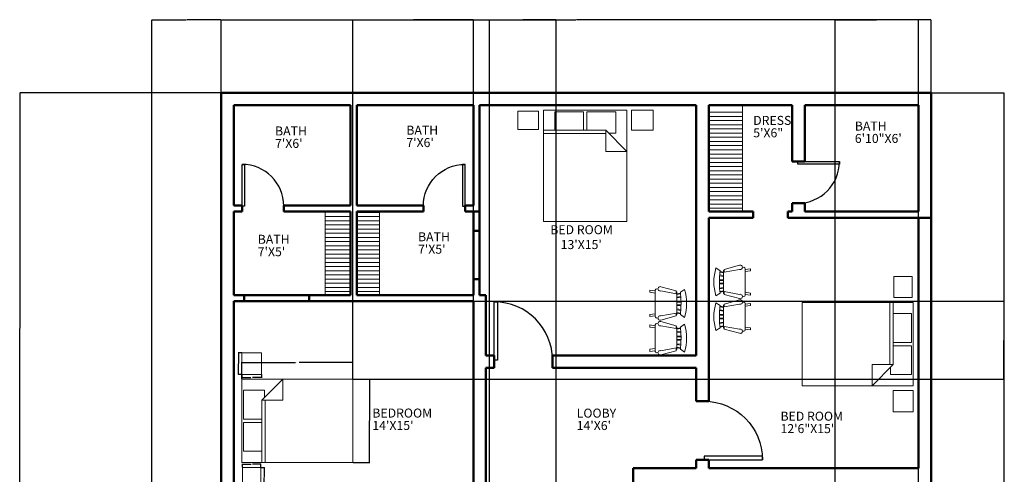
# Model space of a CAD drawing. Units: inches. Extents: x 5375 to 6084, y 16106 to 17259.
# Tile 32 of 32: x 5376 to 6084, y 16932 to 17259. Entities that reach past the tile are written whole.
import ezdxf

# ---------------------------------------------------------------- set-up
doc = ezdxf.new("R2010")
doc.units = ezdxf.units.IN
for name, color, linetype, lineweight in [('A-ANNO-DIMS', 2, 'Continuous', 18), ('A-AREA-IDEN', 5, 'Continuous', 18), ('A-CASE-PATT', 3, 'Continuous', 13), ('A-FLOR-CASE', 3, 'Continuous', 18), ('DOOR', 4, 'Continuous', 25), ('FURNITURE', 3, 'Continuous', 18), ('WALL', 6, 'Continuous', 50)]:
    doc.layers.add(name, color=color, linetype=linetype, lineweight=lineweight)
doc.styles.get("Standard").update_dxf_attribs({"font": 'arial.ttf'})
doc.dimstyles.get("Standard").update_dxf_attribs({"dimtxt": 0.18, "dimasz": 0.18, "dimexe": 0.18, "dimexo": 0.0625, "dimgap": 0.09, "dimtad": 0, "dimtih": 1, "dimtoh": 1, "dimdec": 4, "dimzin": 0, "dimdsep": 46, "dimtxsty": 'Standard', "dimcen": 0.09, "dimadec": 0, "dimazin": 0, "dimtfac": 1, "dimtdec": 4, "dimtofl": 0, "dimtmove": 0, "dimatfit": 3, "dimfxl": 1, "dimtolj": 1, "dimtzin": 0, "dimarcsym": 0})

# ---------------------------------------------------------------- blocks, each defined once
blk = doc.blocks.new('*U2')
for p, q in [((0, 0), (0, -100)), ((750, 0), (750, -100))]:
    blk.add_line(p, q)
blk.add_lwpolyline([(0, 0), (0, 750), (43.75, 750), (43.75, 0)], close=True)
blk.add_arc((0, 0), 750, 0, 90)
blk = doc.blocks.new('Bed - Queen')
for p, q in [((0, -80.00003), (0, 0)), ((0, 0), (59.99999, 0)), ((59.99999, 0), (59.99999, -80.00003)), ((7.99999, -1.2), (28.79998, -1.2)), ((7.99999, -14.4), (7.99999, -1.2)), ((28.79998, -1.2), (28.79998, -14.4)), ((31.19999, -1.2), (51.99999, -1.2)), ((31.19999, -14.4), (31.19999, -1.2)), ((51.99999, -1.2), (51.99999, -16.4)), ((0, -14.4), (44.8, -14.4)), ((44.8, -16.8), (0, -16.8)), ((59.99999, -29.6), (44.8, -14.4)), ((44.8, -14.4), (44.8, -29.6)), ((51.99999, -16.4), (46.79936, -16.4)), ((44.8, -29.6), (59.99999, -29.6)), ((59.99999, -80.00003), (0, -80.00003))]:
    blk.add_line(p, q)
blk = doc.blocks.new('Chair - Rocking')
for p, q in [((-8, -4.5), (-10, -1.5)), ((-8.23428, -6.99939), (-8.3093, -7.47958)), ((-8.23041, -7), (8.23915, -7)), ((-7.5, -4.5), (-7, -7)), ((-6.5, -7), (-7.02225, -4.43)), ((-4.5, -7), (-4.96674, -4.19951)), ((-4, -7), (-4.40532, -4.16272)), ((-1.5, -4.05012), (-1.5, -7)), ((-1, -7), (-1, -4.05012)), ((1, -7), (1, -4.04655)), ((1.5, -4.05012), (1.5, -7)), ((4, -7), (4.40187, -4.18694)), ((4.5, -7), (4.96761, -4.19437)), ((6.5, -7), (7, -4.4057)), ((7.5, -4.5), (7, -7)), ((8, -4.5), (10, -1.5)), ((8.31071, -7.48854), (8.23449, -7.00073)), ((-9, -7.5), (-12, -18.49999)), ((-7, -7.5), (-9, -7.5)), ((-9, -18.49999), (-7, -7.5)), ((7, -7.5), (9, -7.5)), ((9, -18.49999), (7, -7.5)), ((9, -7.5), (12, -18.49999)), ((-10.36644, -20.64523), (-10.5, -21.49999)), ((10.5, -21.49999), (10.3575, -20.58798)), ((-9, -22.49999), (-9.5, -26.49999)), ((0, -22.49999), (-9.5, -22.49999)), ((-9.5, -26.49999), (-8, -26.49999)), ((-8, -26.49999), (-7.5, -22.49999)), ((0, -22.49999), (9.5, -22.49999)), ((8, -26.49999), (7.5, -22.49999)), ((9.5, -26.49999), (8, -26.49999)), ((9, -22.49999), (9.5, -26.49999))]:
    blk.add_line(p, q)
for centre, radius, start, end in [((0, -34.08333), 34.08333, 72.93847, 107.0615), ((0, -68.25004), 64.25, 93.92211, 97.15267), ((0, -68.25004), 64.25, 82.84733, 93.92211), ((-10.5, -18.99999), 1.58114, 161.5651, 18.43495), ((10.5, -18.99999), 1.58114, 161.5651, 18.43495), ((-9.5, -21.49999), 1, 180, 270), ((9.5, -21.49999), 1, 270, 0)]:
    blk.add_arc(centre, radius, start, end)
blk = doc.blocks.new('NIGHTSTAND-SMALL')
blk.add_lwpolyline([(0, 13.23), (15.04, 13.23), (15.04, 0), (0, 0)], close=True)
blk = doc.blocks.new('NIGHTSTAND-LARGE')
blk.add_lwpolyline([(0, 14.27), (15.49, 14.27), (15.49, 0), (0, 0)], close=True)
blk = doc.blocks.new('*D16')
at = {"layer": 'A-ANNO-DIMS', "color": 0, "lineweight": -2, "transparency": 16777216}
for p, q in [((5535.35, 17019.44), (5532.91, 17019.44)), ((5533.09, 17019.26), (5533.09, 17011.88)), ((5533.09, 17004.13), (5533.09, 17011.52)), ((5535.35, 17003.95), (5532.91, 17003.95))]:
    blk.add_line(p, q, dxfattribs=at)
at = {"layer": 'A-ANNO-DIMS', "color": 0, "transparency": 16777216}
for points in [[(5533.06, 17019.26), (5533.12, 17019.26), (5533.09, 17019.44)], [(5533.06, 17004.13), (5533.12, 17004.13), (5533.09, 17003.95)]]:
    blk.add_solid(points, dxfattribs=at)
at = {"layer": 'Defpoints', "color": 0, "transparency": 16777216}
for p in [(5533.09, 17019.44), (5535.41, 17019.44), (5535.41, 17003.95)]:
    blk.add_point(p, dxfattribs=at)
at = {"layer": 'A-ANNO-DIMS', "color": 0, "transparency": 16777216, "insert": (5533.09, 17011.7), "char_height": 0.18, "attachment_point": 5}
blk.add_mtext('\\A1;LG. NIGHTSTAND 15 TYP.', dxfattribs=at)
blk = doc.blocks.new('*D17')
at = {"layer": 'A-ANNO-DIMS', "color": 0, "lineweight": -2, "transparency": 16777216}
for p, q in [((5535.41, 17003.89), (5535.41, 17001.45)), ((5549.68, 17003.89), (5549.68, 17001.45)), ((5535.59, 17001.63), (5542.03, 17001.63)), ((5549.5, 17001.63), (5543.07, 17001.63))]:
    blk.add_line(p, q, dxfattribs=at)
at = {"layer": 'A-ANNO-DIMS', "color": 0, "transparency": 16777216}
for points in [[(5535.59, 17001.66), (5535.59, 17001.6), (5535.41, 17001.63)], [(5549.5, 17001.66), (5549.5, 17001.6), (5549.68, 17001.63)]]:
    blk.add_solid(points, dxfattribs=at)
at = {"layer": 'Defpoints', "color": 0, "transparency": 16777216}
for p in [(5535.41, 17003.95), (5549.68, 17003.95), (5535.41, 17001.63)]:
    blk.add_point(p, dxfattribs=at)
at = {"layer": 'A-ANNO-DIMS', "color": 0, "transparency": 16777216, "insert": (5542.55, 17001.63), "char_height": 0.18, "attachment_point": 5}
blk.add_mtext('\\A1;14 TYP.', dxfattribs=at)
blk = doc.blocks.new('*D18')
at = {"layer": 'A-ANNO-DIMS', "color": 0, "lineweight": -2, "transparency": 16777216}
for p, q in [((5549.3, 16937.05), (5551.67, 16937.05)), ((5551.49, 16936.87), (5551.49, 16929.72)), ((5551.49, 16922.19), (5551.49, 16929.35)), ((5549.3, 16922.01), (5551.67, 16922.01))]:
    blk.add_line(p, q, dxfattribs=at)
at = {"layer": 'A-ANNO-DIMS', "color": 0, "transparency": 16777216}
for points in [[(5551.46, 16936.87), (5551.52, 16936.87), (5551.49, 16937.05)], [(5551.46, 16922.19), (5551.52, 16922.19), (5551.49, 16922.01)]]:
    blk.add_solid(points, dxfattribs=at)
at = {"layer": 'Defpoints', "color": 0, "transparency": 16777216}
for p in [(5549.24, 16937.05), (5551.49, 16937.05), (5549.24, 16922.01)]:
    blk.add_point(p, dxfattribs=at)
at = {"layer": 'A-ANNO-DIMS', "color": 0, "transparency": 16777216, "insert": (5551.49, 16929.53), "char_height": 0.18, "attachment_point": 5}
blk.add_mtext('\\A1;SM. NIGHTSTAND 15 TYP.', dxfattribs=at)
blk = doc.blocks.new('*D19')
at = {"layer": 'A-ANNO-DIMS', "color": 0, "lineweight": -2, "transparency": 16777216}
for p, q in [((5536.01, 16937.12), (5536.01, 16939.49)), ((5536.19, 16939.31), (5542.1, 16939.31)), ((5549.06, 16939.31), (5543.14, 16939.31)), ((5549.24, 16937.12), (5549.24, 16939.49))]:
    blk.add_line(p, q, dxfattribs=at)
at = {"layer": 'A-ANNO-DIMS', "color": 0, "transparency": 16777216}
for points in [[(5536.19, 16939.34), (5536.19, 16939.28), (5536.01, 16939.31)], [(5549.06, 16939.34), (5549.06, 16939.28), (5549.24, 16939.31)]]:
    blk.add_solid(points, dxfattribs=at)
at = {"layer": 'Defpoints', "color": 0, "transparency": 16777216}
for p in [(5536.01, 16939.31), (5536.01, 16937.05), (5549.24, 16937.05)]:
    blk.add_point(p, dxfattribs=at)
at = {"layer": 'A-ANNO-DIMS', "color": 0, "transparency": 16777216, "insert": (5542.62, 16939.31), "char_height": 0.18, "attachment_point": 5}
blk.add_mtext('\\A1;13 TYP.', dxfattribs=at)
blk = doc.blocks.new('*D20')
at = {"layer": 'A-ANNO-DIMS', "color": 0, "lineweight": -2, "transparency": 16777216}
for p, q in [((5535.41, 17000.67), (5535.41, 17012.79)), ((5535.59, 17012.61), (5574.11, 17012.61)), ((5615.23, 17012.61), (5576.72, 17012.61)), ((5615.41, 17000.67), (5615.41, 17012.79))]:
    blk.add_line(p, q, dxfattribs=at)
at = {"layer": 'A-ANNO-DIMS', "color": 0, "transparency": 16777216}
for points in [[(5535.59, 17012.64), (5535.59, 17012.58), (5535.41, 17012.61)], [(5615.23, 17012.64), (5615.23, 17012.58), (5615.41, 17012.61)]]:
    blk.add_solid(points, dxfattribs=at)
at = {"layer": 'Defpoints', "color": 0, "transparency": 16777216}
for p in [(5535.41, 17012.61), (5535.41, 17000.61), (5615.41, 17000.61)]:
    blk.add_point(p, dxfattribs=at)
at = {"layer": 'A-ANNO-DIMS', "color": 0, "transparency": 16777216, "insert": (5575.41, 17012.61), "char_height": 0.18, "attachment_point": 5}
blk.add_mtext('\\A1;QUEEN BED 80 TYP.', dxfattribs=at)
blk = doc.blocks.new('*D21')
at = {"layer": 'A-ANNO-DIMS', "color": 0, "lineweight": -2, "transparency": 16777216}
for p, q in [((5615.48, 17000.61), (5627.59, 17000.61)), ((5627.41, 17000.43), (5627.41, 16970.79)), ((5627.41, 16940.79), (5627.41, 16970.43)), ((5615.48, 16940.61), (5627.59, 16940.61))]:
    blk.add_line(p, q, dxfattribs=at)
at = {"layer": 'A-ANNO-DIMS', "color": 0, "transparency": 16777216}
for points in [[(5627.38, 17000.43), (5627.44, 17000.43), (5627.41, 17000.61)], [(5627.38, 16940.79), (5627.44, 16940.79), (5627.41, 16940.61)]]:
    blk.add_solid(points, dxfattribs=at)
at = {"layer": 'Defpoints', "color": 0, "transparency": 16777216}
for p in [(5615.41, 17000.61), (5627.41, 17000.61), (5615.41, 16940.61)]:
    blk.add_point(p, dxfattribs=at)
at = {"layer": 'A-ANNO-DIMS', "color": 0, "transparency": 16777216, "insert": (5627.41, 16970.61), "char_height": 0.18, "attachment_point": 5}
blk.add_mtext('\\A1;60 TYP.', dxfattribs=at)
blk = doc.blocks.new('*D31')
at = {"layer": 'A-ANNO-DIMS', "color": 0, "lineweight": -2, "transparency": 16777216}
for p, q in [((6031.68, 17206.58), (6084.2, 17206.58)), ((6084.02, 17206.4), (6084.02, 16709.66)), ((6084.02, 16212.56), (6084.02, 16709.3)), ((6031.68, 16212.38), (6084.2, 16212.38))]:
    blk.add_line(p, q, dxfattribs=at)
at = {"layer": 'A-ANNO-DIMS', "color": 0, "transparency": 16777216}
for points in [[(6083.99, 17206.4), (6084.05, 17206.4), (6084.02, 17206.58)], [(6083.99, 16212.56), (6084.05, 16212.56), (6084.02, 16212.38)]]:
    blk.add_solid(points, dxfattribs=at)
at = {"layer": 'Defpoints', "color": 0, "transparency": 16777216}
for p in [(6031.62, 17206.58), (6084.02, 17206.58), (6031.62, 16212.38)]:
    blk.add_point(p, dxfattribs=at)
at = {"layer": 'A-ANNO-DIMS', "color": 0, "transparency": 16777216, "insert": (6084.02, 16709.48), "char_height": 0.18, "attachment_point": 5}
blk.add_mtext('\\A1;994.2', dxfattribs=at)
blk = doc.blocks.new('*D32')
at = {"layer": 'A-ANNO-DIMS', "color": 0, "lineweight": -2, "transparency": 16777216}
for p, q in [((5520.62, 17206.64), (5520.62, 17259.16)), ((6031.62, 17206.64), (6031.62, 17259.16)), ((5520.8, 17258.98), (5775.85, 17258.98)), ((6031.44, 17258.98), (5776.39, 17258.98))]:
    blk.add_line(p, q, dxfattribs=at)
at = {"layer": 'A-ANNO-DIMS', "color": 0, "transparency": 16777216}
for points in [[(5520.8, 17259.01), (5520.8, 17258.95), (5520.62, 17258.98)], [(6031.44, 17259.01), (6031.44, 17258.95), (6031.62, 17258.98)]]:
    blk.add_solid(points, dxfattribs=at)
at = {"layer": 'Defpoints', "color": 0, "transparency": 16777216}
for p in [(6031.62, 17258.98), (5520.62, 17206.58), (6031.62, 17206.58)]:
    blk.add_point(p, dxfattribs=at)
at = {"layer": 'A-ANNO-DIMS', "color": 0, "transparency": 16777216, "insert": (5776.12, 17258.98), "char_height": 0.18, "attachment_point": 5}
blk.add_mtext('\\A1;511', dxfattribs=at)
blk = doc.blocks.new('*D37')
at = {"layer": 'A-ANNO-DIMS', "color": 0, "lineweight": -2, "transparency": 16777216}
for p, q in [((5520.56, 17206.58), (5375.56, 17206.58)), ((5375.74, 17206.4), (5375.74, 17037.26)), ((5375.74, 16867.76), (5375.74, 17036.9)), ((5520.56, 16867.58), (5375.56, 16867.58))]:
    blk.add_line(p, q, dxfattribs=at)
at = {"layer": 'A-ANNO-DIMS', "color": 0, "transparency": 16777216}
for points in [[(5375.71, 17206.4), (5375.77, 17206.4), (5375.74, 17206.58)], [(5375.71, 16867.76), (5375.77, 16867.76), (5375.74, 16867.58)]]:
    blk.add_solid(points, dxfattribs=at)
at = {"layer": 'Defpoints', "color": 0, "transparency": 16777216}
for p in [(5375.74, 17206.58), (5520.62, 17206.58), (5520.62, 16867.58)]:
    blk.add_point(p, dxfattribs=at)
at = {"layer": 'A-ANNO-DIMS', "color": 0, "transparency": 16777216, "insert": (5375.74, 17037.08), "char_height": 0.18, "attachment_point": 5}
blk.add_mtext('\\A1;339', dxfattribs=at)
blk = doc.blocks.new('*D39')
at = {"layer": 'A-ANNO-DIMS', "color": 0, "lineweight": -2, "transparency": 16777216}
for p, q in [((5713.62, 16402.64), (5713.62, 17259.16)), ((5761.62, 16402.64), (5761.62, 17259.16)), ((5713.8, 17258.98), (5737.4, 17258.98)), ((5761.44, 17258.98), (5737.84, 17258.98))]:
    blk.add_line(p, q, dxfattribs=at)
at = {"layer": 'A-ANNO-DIMS', "color": 0, "transparency": 16777216}
for points in [[(5713.8, 17259.01), (5713.8, 17258.95), (5713.62, 17258.98)], [(5761.44, 17259.01), (5761.44, 17258.95), (5761.62, 17258.98)]]:
    blk.add_solid(points, dxfattribs=at)
at = {"layer": 'Defpoints', "color": 0, "transparency": 16777216}
for p in [(5761.62, 17258.98), (5713.62, 16402.58), (5761.62, 16402.58)]:
    blk.add_point(p, dxfattribs=at)
at = {"layer": 'A-ANNO-DIMS', "color": 0, "transparency": 16777216, "insert": (5737.62, 17258.98), "char_height": 0.18, "attachment_point": 5}
blk.add_mtext('\\A1;48', dxfattribs=at)
blk = doc.blocks.new('*D47')
at = {"layer": 'A-ANNO-DIMS', "color": 0, "lineweight": -2, "transparency": 16777216}
for p, q in [((5470.62, 16603.64), (5470.62, 17259.16)), ((5520.62, 17206.64), (5520.62, 17259.16)), ((5470.8, 17258.98), (5495.4, 17258.98)), ((5520.44, 17258.98), (5495.84, 17258.98))]:
    blk.add_line(p, q, dxfattribs=at)
at = {"layer": 'A-ANNO-DIMS', "color": 0, "transparency": 16777216}
for points in [[(5470.8, 17259.01), (5470.8, 17258.95), (5470.62, 17258.98)], [(5520.44, 17259.01), (5520.44, 17258.95), (5520.62, 17258.98)]]:
    blk.add_solid(points, dxfattribs=at)
at = {"layer": 'Defpoints', "color": 0, "transparency": 16777216}
for p in [(5520.62, 17258.98), (5520.62, 17206.58), (5470.62, 16603.58)]:
    blk.add_point(p, dxfattribs=at)
at = {"layer": 'A-ANNO-DIMS', "color": 0, "transparency": 16777216, "insert": (5495.62, 17258.98), "char_height": 0.18, "attachment_point": 5}
blk.add_mtext('\\A1;50', dxfattribs=at)
blk = doc.blocks.new('*D48')
at = {"layer": 'A-ANNO-DIMS', "color": 0, "lineweight": -2, "transparency": 16777216}
for p, q in [((5962.62, 16411.64), (5962.62, 17259.16)), ((6022.62, 16411.64), (6022.62, 17259.16)), ((5962.8, 17258.98), (5992.4, 17258.98)), ((6022.44, 17258.98), (5992.84, 17258.98))]:
    blk.add_line(p, q, dxfattribs=at)
at = {"layer": 'A-ANNO-DIMS', "color": 0, "transparency": 16777216}
for points in [[(5962.8, 17259.01), (5962.8, 17258.95), (5962.62, 17258.98)], [(6022.44, 17259.01), (6022.44, 17258.95), (6022.62, 17258.98)]]:
    blk.add_solid(points, dxfattribs=at)
at = {"layer": 'Defpoints', "color": 0, "transparency": 16777216}
for p in [(6022.62, 17258.98), (5962.62, 16411.58), (6022.62, 16411.58)]:
    blk.add_point(p, dxfattribs=at)
at = {"layer": 'A-ANNO-DIMS', "color": 0, "transparency": 16777216, "insert": (5992.62, 17258.98), "char_height": 0.18, "attachment_point": 5}
blk.add_mtext('\\A1;60', dxfattribs=at)
blk = doc.blocks.new('*D49')
at = {"layer": 'A-ANNO-DIMS', "color": 0, "lineweight": -2, "transparency": 16777216}
for p, q in [((5529.68, 17056.58), (6084.2, 17056.58)), ((6084.02, 17056.4), (6084.02, 17028.78)), ((6084.02, 17000.79), (6084.02, 17028.41)), ((5615.48, 17000.61), (6084.2, 17000.61))]:
    blk.add_line(p, q, dxfattribs=at)
at = {"layer": 'A-ANNO-DIMS', "color": 0, "transparency": 16777216}
for points in [[(6083.99, 17056.4), (6084.05, 17056.4), (6084.02, 17056.58)], [(6083.99, 17000.79), (6084.05, 17000.79), (6084.02, 17000.61)]]:
    blk.add_solid(points, dxfattribs=at)
at = {"layer": 'Defpoints', "color": 0, "transparency": 16777216}
for p in [(5529.62, 17056.58), (5615.41, 17000.61), (6084.02, 17000.61)]:
    blk.add_point(p, dxfattribs=at)
at = {"layer": 'A-ANNO-DIMS', "color": 0, "transparency": 16777216, "insert": (6084.02, 17028.59), "char_height": 0.18, "attachment_point": 5}
blk.add_mtext('\\A1;55.97', dxfattribs=at)
blk = doc.blocks.new('*D50')
at = {"layer": 'A-ANNO-DIMS', "color": 0, "lineweight": -2, "transparency": 16777216}
for p, q in [((5615.41, 17000.67), (5615.41, 17259.16)), ((5702.12, 17056.64), (5702.12, 17259.16)), ((5615.59, 17258.98), (5658.44, 17258.98)), ((5701.94, 17258.98), (5659.09, 17258.98))]:
    blk.add_line(p, q, dxfattribs=at)
at = {"layer": 'A-ANNO-DIMS', "color": 0, "transparency": 16777216}
for points in [[(5615.59, 17259.01), (5615.59, 17258.95), (5615.41, 17258.98)], [(5701.94, 17259.01), (5701.94, 17258.95), (5702.12, 17258.98)]]:
    blk.add_solid(points, dxfattribs=at)
at = {"layer": 'Defpoints', "color": 0, "transparency": 16777216}
for p in [(5702.12, 17258.98), (5702.12, 17056.58), (5615.41, 17000.61)]:
    blk.add_point(p, dxfattribs=at)
at = {"layer": 'A-ANNO-DIMS', "color": 0, "transparency": 16777216, "insert": (5658.77, 17258.98), "char_height": 0.18, "attachment_point": 5}
blk.add_mtext('\\A1;86.7', dxfattribs=at)

msp = doc.modelspace()

# ---------------------------------------------------------------- hatches: boundary and pattern name
at = {"layer": 'A-CASE-PATT'}
h = msp.add_hatch(dxfattribs=at)
h.set_pattern_fill('ANSI31', color=256, scale=0.944856, angle=-45, style=0)
h.paths.add_polyline_path([(5871.6199, 17122.0277), (5895.7926, 17122.0277), (5895.7926, 17194.0277), (5871.6199, 17194.0277)])
h = msp.add_hatch(dxfattribs=at)
h.set_pattern_fill('ANSI31', color=256, scale=0.9448558, angle=-45, style=0)
h.paths.add_polyline_path([(5595.4235, 17062.046), (5613.6199, 17062.046), (5613.6199, 17119.0277), (5595.4235, 17119.0277)])
h = msp.add_hatch(dxfattribs=at)
h.set_pattern_fill('ANSI31', color=256, scale=0.9448558, angle=-45, style=0)
h.paths.add_polyline_path([(5618.1199, 17061.5998), (5634.4811, 17061.5998), (5634.4811, 17121.0793), (5618.1199, 17121.0793)])

# ---------------------------------------------------------------- linework, layer by layer
at = {"layer": 'A-FLOR-CASE'}
for p, q in [((5895.7926, 17121.0793), (5895.7926, 17197.5793)), ((5595.4235, 17061.0793), (5595.4235, 17121.0793)), ((5634.4811, 17061.0793), (5634.4811, 17121.0793))]:
    msp.add_line(p, q, dxfattribs=at)
at = {"layer": 'WALL'}
for p, q in [((5520.6199, 17206.5793), (6031.6199, 17206.5793)), ((5520.6199, 17206.5793), (5520.6199, 16867.5793)), ((6031.6199, 17206.5793), (6031.6199, 16921.5793)), ((5529.6199, 17197.5793), (5613.6199, 17197.5793)), ((5529.6199, 17197.5793), (5529.6199, 17125.5793)), ((5613.6199, 17197.5793), (5613.6199, 17125.5793)), ((5618.1199, 17197.5793), (5618.1199, 17125.5793)), ((5618.1199, 17197.5793), (5702.1199, 17197.5793)), ((5702.1199, 17197.5793), (5702.1199, 17125.5793)), ((5706.6199, 17197.5793), (5706.6199, 17061.0793)), ((5706.6199, 17197.5793), (5862.6199, 17197.5793)), ((5862.6199, 17197.5793), (5862.6199, 17017.5793)), ((5871.6199, 17197.5793), (5871.6199, 17121.0793)), ((5871.6199, 17197.5793), (5931.6199, 17197.5793)), ((5931.6199, 17197.5793), (5931.6199, 17157.0793)), ((5940.6199, 17197.5793), (5940.6199, 17157.0793)), ((5940.6199, 17197.5793), (6022.6199, 17197.5793)), ((6022.6199, 17197.5793), (6022.6199, 17121.0793)), ((5931.6199, 17157.0793), (5940.6199, 17157.0793)), ((5529.6199, 17125.5793), (5535.6199, 17125.5793)), ((5535.6199, 17125.5793), (5535.6199, 17121.0793)), ((5565.6199, 17125.5793), (5565.6199, 17121.0793)), ((5565.6199, 17125.5793), (5613.6199, 17125.5793)), ((5618.1199, 17125.5793), (5666.1199, 17125.5793)), ((5666.1199, 17125.5793), (5666.1199, 17121.0793)), ((5696.1199, 17125.5793), (5696.1199, 17121.0793)), ((5696.1199, 17125.5793), (5702.1199, 17125.5793)), ((5931.6199, 17127.0793), (5940.6199, 17127.0793)), ((5931.6199, 17127.0793), (5931.6199, 17121.0793)), ((5940.6199, 17127.0793), (5940.6199, 17121.0793)), ((5529.6199, 17121.0793), (5535.6199, 17121.0793)), ((5529.6199, 17121.0793), (5529.6199, 17061.0793)), ((5565.6199, 17121.0793), (5613.6199, 17121.0793)), ((5613.6199, 17121.0793), (5613.6199, 17061.0793)), ((5618.1199, 17121.0793), (5618.1199, 17061.0793)), ((5618.1199, 17121.0793), (5666.1199, 17121.0793)), ((5696.1199, 17121.0793), (5706.6199, 17121.0793)), ((5702.1199, 17121.0793), (5702.1199, 17061.0793)), ((5871.6199, 17121.0793), (5903.5874, 17121.0793)), ((5903.5874, 17116.5793), (5903.5874, 17121.0793)), ((5928.429, 17116.5793), (5928.429, 17121.0793)), ((5928.429, 17121.0793), (5931.6199, 17121.0793)), ((5940.6199, 17121.0793), (6022.6199, 17121.0793)), ((5871.6199, 17116.5793), (5903.5874, 17116.5793)), ((5871.6199, 17116.5793), (5871.6199, 16984.5793)), ((5928.429, 17116.5793), (6031.6199, 17116.5793)), ((6022.6199, 17116.5793), (6022.6199, 16936.5793)), ((5702.1199, 17107.1519), (5706.6199, 17107.1519)), ((5702.1199, 17072.3648), (5706.6199, 17072.3648)), ((5529.6199, 17061.0793), (5613.6199, 17061.0793)), ((5537.0821, 17056.5793), (5537.0821, 17061.0793)), ((5583.9756, 17056.5793), (5583.9756, 17061.0793)), ((5618.1199, 17061.0793), (5702.1199, 17061.0793)), ((5706.6199, 17061.0793), (5711.1199, 17061.0793)), ((5711.1199, 17061.0793), (5711.1199, 17017.5793)), ((5529.6199, 17056.5793), (5702.1199, 17056.5793)), ((5529.6199, 17056.5793), (5529.6199, 16876.5793)), ((5618.1199, 17056.5793), (5702.1199, 17056.5793)), ((5702.1199, 17056.5793), (5702.1199, 16924.5793)), ((5711.1199, 17017.5793), (5717.1199, 17017.5793)), ((5717.1199, 17017.5793), (5717.1199, 17008.5793)), ((5759.1199, 17017.5793), (5759.1199, 17008.5793)), ((5759.1199, 17017.5793), (5862.6199, 17017.5793)), ((5711.1199, 17008.5793), (5717.1199, 17008.5793)), ((5711.1199, 17008.5793), (5711.1199, 16924.5793)), ((5759.1199, 17008.5793), (5862.6199, 17008.5793)), ((5862.6199, 17008.5793), (5862.6199, 16984.5793)), ((5862.6199, 16984.5793), (5871.6199, 16984.5793)), ((5862.6199, 16942.5793), (5871.6199, 16942.5793)), ((5862.6199, 16942.5793), (5862.6199, 16936.5793)), ((5871.6199, 16942.5793), (5871.6199, 16936.5793)), ((5817.1199, 16936.5793), (5862.6199, 16936.5793)), ((5817.1199, 16936.5793), (5817.1199, 16921.5793)), ((5871.6199, 16936.5793), (6022.6199, 16936.5793))]:
    msp.add_line(p, q, dxfattribs=at)

# ---------------------------------------------------------------- block references
at = {"layer": 'DOOR'}
for p, xscale, yscale, zscale in [((5535.6199, 17125.0793), 0.0399999999999999, 0.0399999999999999, 0.0399999999999999), ((5696.1199, 17125.0793), -0.0399999999999999, 0.0399999999999999, 0.0399999999999999), ((5717.1199, 17014.1793), 0.0559999999999998, 0.0559999999999998, 0.0559999999999998)]:
    msp.add_blockref('*U2', p, dxfattribs=dict(at, xscale=xscale, yscale=yscale, zscale=zscale))
at = {"layer": 'DOOR', "rotation": 270}
for p, xscale, yscale, zscale in [((5935.6199, 17157.0793), 0.0399999999999999, 0.0399999999999999, 0.0399999999999999), ((5868.2199, 16942.5793), -0.0559999999999998, 0.0559999999999998, 0.0559999999999998)]:
    msp.add_blockref('*U2', p, dxfattribs=dict(at, xscale=xscale, yscale=yscale, zscale=zscale))
at = {"layer": 'FURNITURE'}
for name, p in [('NIGHTSTAND-SMALL', (5734.075, 17180.154)), ('Bed - Queen', (5752.6728, 17193.9756)), ('NIGHTSTAND-LARGE', (5816.018, 17179.706))]:
    msp.add_blockref(name, p, dxfattribs=at)
at = {"layer": 'FURNITURE', "xscale": -1, "rotation": 90}
for p in [(5875.2273, 17070.5124), (5875.2273, 17045.5147)]:
    msp.add_blockref('Chair - Rocking', p, dxfattribs=at)
at = {"layer": 'FURNITURE'}
for name, p, rotation in [('NIGHTSTAND-SMALL', (6004.8863, 17074.3998), 269.999999999987), ('Chair - Rocking', (5855.6126, 17055.0147), 270), ('Bed - Queen', (6018.7079, 17055.802), 270), ('Chair - Rocking', (5855.6126, 17030.0169), 270), ('NIGHTSTAND-LARGE', (5549.6843, 17003.9546), 89.9999999999909), ('Bed - Queen', (5535.4147, 16940.6094), 90), ('NIGHTSTAND-LARGE', (6004.4383, 16992.4568), 269.9999999999879), ('NIGHTSTAND-SMALL', (5549.2363, 16922.0116), 89.99999999998697)]:
    msp.add_blockref(name, p, dxfattribs=dict(at, rotation=rotation))

# ---------------------------------------------------------------- texts
at = {"layer": 'A-AREA-IDEN'}
for s, p in [('DRESS', (5903.5802, 17183.4608)), ('BATH', (5559.3831, 17175.8637)), ('BATH', (5653.8753, 17176.4408)), ('5\'X6"', (5903.5802, 17174.5277)), ('BATH', (5976.7182, 17179.4199)), ("7'X6'", (5653.8753, 17167.5077)), ('6\'10"X6\'', (5976.7182, 17170.4868)), ("7'X6'", (5559.3831, 17166.9306)), ('BED ROOM', (5757.5117, 17104.8291)), ('BATH', (5546.9143, 17097.9208)), ('BATH', (5662.3043, 17099.7311)), ("7'X5'", (5662.3043, 17090.798)), ("13'X15'", (5764.9716, 17094.1314)), ("7'X5'", (5546.9143, 17088.9878)), ('BEDROOM', (5629.4173, 16972.8993)), ('LOOBY', (5776.5095, 16972.8578)), ('BED ROOM', (5923.2301, 16970.6516)), ("14'X15'", (5629.4173, 16963.9663)), ("14'X6'", (5776.5095, 16963.9247)), ('12\'6"X15\'', (5923.2301, 16961.7186))]:
    msp.add_text(s, height=6.47981, dxfattribs=at).set_placement(p)

# ---------------------------------------------------------------- dimensions: what is measured, and where the dimension line sits
at = {"layer": 'A-ANNO-DIMS'}
for base, p1, p2, override, picture, middle in [((5520.6199, 17258.9793), (5470.6199, 16603.5793), (5520.6199, 17206.5793), {"dimdec": 0, "dimlfac": 1, "dimrnd": 0, "dimzin": 0, "dimdsep": 46, "dimlunit": 2}, '*D47', (5495.6199, 17258.9793)), ((6031.6199, 17258.9793), (5520.6199, 17206.5793), (6031.6199, 17206.5793), {"dimdec": 0, "dimlfac": 1, "dimrnd": 0, "dimzin": 0, "dimdsep": 46, "dimlunit": 2}, '*D32', (5776.1199, 17258.9793)), ((5702.1199, 17258.9793), (5615.4147, 17000.6094), (5702.1199, 17056.5793), {"dimdec": 1, "dimlfac": 1, "dimrnd": 0, "dimzin": 0, "dimdsep": 46, "dimlunit": 2}, '*D50', (5658.7673, 17258.9793)), ((5761.6199, 17258.9793), (5713.6199, 16402.5793), (5761.6199, 16402.5793), {"dimdec": 0, "dimlfac": 1, "dimrnd": 0, "dimzin": 0, "dimdsep": 46, "dimlunit": 2}, '*D39', (5737.6199, 17258.9793)), ((6022.6199, 17258.9793), (5962.6199, 16411.5793), (6022.6199, 16411.5793), {"dimdec": 0, "dimlfac": 1, "dimrnd": 0, "dimzin": 0, "dimdsep": 46, "dimlunit": 2}, '*D48', (5992.6199, 17258.9793))]:
    dim = msp.add_linear_dim(base=base, p1=p1, p2=p2, dimstyle='Standard', override=override, dxfattribs=at)
    dim.commit()
    dim.dimension.update_dxf_attribs({"geometry": picture, "text_midpoint": middle})
for base, p1, p2, override, picture, middle in [((5375.7423, 17206.5793), (5520.6199, 16867.5793), (5520.6199, 17206.5793), {"dimdec": 0, "dimlfac": 1, "dimrnd": 0, "dimzin": 0, "dimdsep": 46, "dimlunit": 2}, '*D37', (5375.7423, 17037.0793)), ((6084.0199, 17206.5793), (6031.6199, 16212.3785), (6031.6199, 17206.5793), {"dimdec": 1, "dimlfac": 1, "dimrnd": 0, "dimzin": 0, "dimdsep": 46, "dimlunit": 2}, '*D31', (6084.0199, 16709.4789)), ((6084.0199, 17000.6094), (5529.6199, 17056.5793), (5615.4147, 17000.6094), {"dimdec": 2, "dimlfac": 1, "dimrnd": 0, "dimzin": 0, "dimdsep": 46, "dimlunit": 2}, '*D49', (6084.0199, 17028.5943))]:
    dim = msp.add_linear_dim(base=base, p1=p1, p2=p2, angle=90, dimstyle='Standard', override=override, dxfattribs=at)
    dim.commit()
    dim.dimension.update_dxf_attribs({"geometry": picture, "text_midpoint": middle})
for base, p1, p2, angle, text, picture, middle in [((5533.0911, 17019.445), (5535.4147, 17003.9543), (5535.4147, 17019.445), 90, 'LG. NIGHTSTAND <> TYP.', '*D16', (5533.0911, 17011.6997)), ((5535.4147, 17012.6094), (5615.4147, 17000.6094), (5535.4147, 17000.6094), 180, 'QUEEN BED <> TYP.', '*D20', (5575.4147, 17012.6094)), ((5535.4147, 17001.6308), (5549.6843, 17003.9543), (5535.4147, 17003.9543), 180, '<> TYP.', '*D17', (5542.5495, 17001.6308)), ((5627.4148, 17000.6094), (5615.4147, 16940.6094), (5615.4147, 17000.6094), 90, '<> TYP.', '*D21', (5627.4148, 16970.6094)), ((5536.0062, 16939.3094), (5549.2359, 16937.0532), (5536.0062, 16937.0532), 180, '<> TYP.', '*D19', (5542.6211, 16939.3094)), ((5551.4921, 16937.0532), (5549.2359, 16922.0117), (5549.2359, 16937.0532), 90, 'SM. NIGHTSTAND <> TYP.', '*D18', (5551.4921, 16929.5324))]:
    dim = msp.add_linear_dim(base=base, p1=p1, p2=p2, angle=angle, text=text, dimstyle='Standard', override={"dimdec": 0, "dimlfac": 1, "dimrnd": 0, "dimzin": 0, "dimdsep": 46, "dimlunit": 2}, dxfattribs=at)
    dim.commit()
    dim.dimension.update_dxf_attribs({"geometry": picture, "text_midpoint": middle})

doc.saveas('drawing.dxf')
